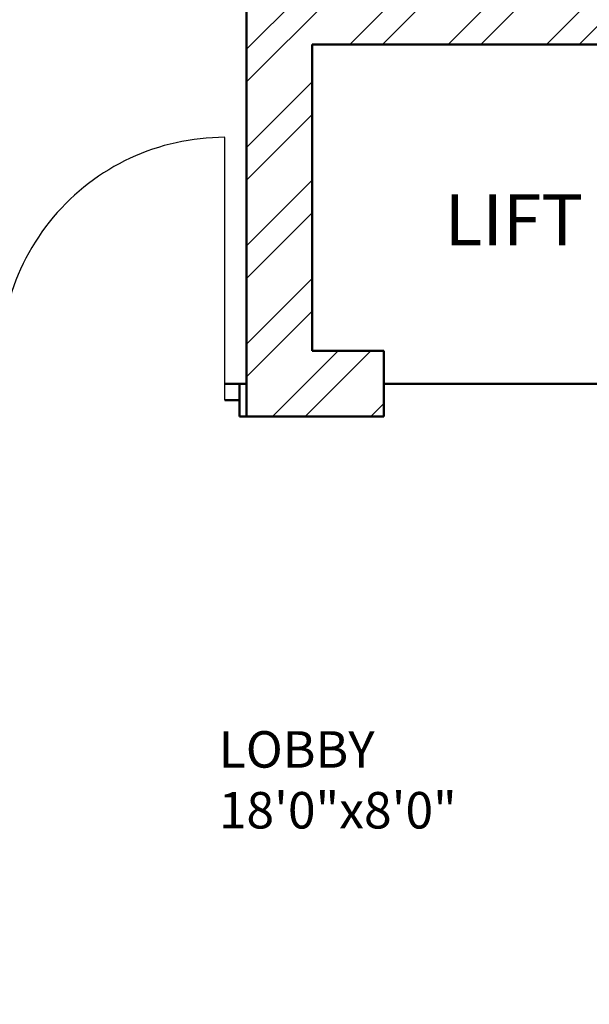
# Model space of a CAD drawing. Units: inches. Extents: x 1901 to 2863, y 888 to 2433.
# Tile 52 of 91: x 2303 to 2381, y 1732 to 1867. Entities that reach past the tile are written whole.
import ezdxf

# ---------------------------------------------------------------- set-up
doc = ezdxf.new("R2010")
doc.units = ezdxf.units.IN
for name, color, linetype, lineweight in [('A-AREA-IDEN', 7, 'Continuous', 18), ('A-DOOR', 4, 'Continuous', 25), ('A-WALL', 7, 'Continuous', 50), ('A-WALL-PATT', 8, 'Continuous', 13)]:
    doc.layers.add(name, color=color, linetype=linetype, lineweight=lineweight)
doc.styles.get("Standard").update_dxf_attribs({"font": 'arial.ttf'})

msp = doc.modelspace()

# ---------------------------------------------------------------- hatches: boundary and pattern name
at = {"layer": 'A-WALL-PATT'}
h = msp.add_hatch(dxfattribs=at)
h.set_pattern_fill('ANSI32', color=256)
h.paths.add_polyline_path([(2192.5, 2274.13), (2141.26, 2274.13), (2141.26, 2269.63), (2192.5, 2269.63)])
h.paths.add_polyline_path([(2259.93, 2274.13), (2216.5, 2274.13), (2216.5, 2269.63), (2255.43, 2269.63), (2255.43, 2214.63), (2250.81, 2214.63), (2250.81, 2210.13), (2259.93, 2210.13), (2259.93, 2215.13), (2271.76, 2215.13), (2271.76, 2217.38), (2271.76, 2219.63), (2259.93, 2219.63)])
h.paths.add_polyline_path([(2171.43, 2269.63), (2166.93, 2269.63), (2166.93, 2219.63), (2121.24, 2219.63), (2121.24, 2215.13), (2166.93, 2215.13), (2166.93, 2083.13), (2161.81, 2083.13), (2161.81, 2078.63), (2171.43, 2078.63), (2177, 2078.63), (2177, 2080.88), (2177, 2083.13), (2171.43, 2083.13), (2171.43, 2210.13), (2230.91, 2210.13), (2230.91, 2212.38), (2230.91, 2214.63), (2171.43, 2214.63)])
h.paths.add_polyline_path([(2117.26, 2274.13), (2089.43, 2274.13), (2089.43, 2219.63), (2081.14, 2219.63), (2081.14, 2215.13), (2089.43, 2215.13), (2098, 2215.13), (2098, 2217.38), (2098, 2219.63), (2093.93, 2219.63), (2093.93, 2269.63), (2117.26, 2269.63), (2117.26, 2271.88)])
h.paths.add_polyline_path([(2343.43, 2219.63), (2329.29, 2219.63), (2329.29, 2215.13), (2338.93, 2215.13), (2338.93, 2184.74), (2343.43, 2184.74)])
h.paths.add_polyline_path([(2338.93, 2083.13), (2329.29, 2083.13), (2208.97, 2083.13), (2208.97, 2078.63), (2338.93, 2078.63)])
h.paths.add_polyline_path([(2343.43, 2136.74), (2338.93, 2136.74), (2338.93, 1872.63), (2343.43, 1872.63)])
h.paths.add_polyline_path([(2343.43, 1863.63), (2397.68, 1863.63), (2397.68, 1821.63), (2384.14, 1821.63), (2384.14, 1812.63), (2418.33, 1812.63), (2418.33, 1817.13), (2418.33, 1821.63), (2406.68, 1821.63), (2406.68, 1863.63), (2459.5, 1863.63), (2459.5, 1821.63), (2447.14, 1821.63), (2447.14, 1812.63), (2459.5, 1812.63), (2468.5, 1812.63), (2468.5, 1872.63), (2394.43, 1872.63), (2334.43, 1872.63), (2334.43, 1812.63), (2343.43, 1812.63), (2353.25, 1812.63), (2353.25, 1821.63), (2343.43, 1821.63)])
h.paths.add_polyline_path([(2510.01, 1872.63), (2468.5, 1872.63), (2468.5, 1868.13), (2510.01, 1868.13)])
h.paths.add_polyline_path([(2514.01, 1817.13), (2468.5, 1817.13), (2468.5, 1812.63), (2482.11, 1812.63), (2482.11, 1800.61), (2486.61, 1800.61), (2486.61, 1812.63), (2514.01, 1812.63)])
h.paths.add_polyline_path([(2299.25, 1814.88), (2299.25, 1817.13), (2295.93, 1817.13), (2295.93, 1854.17), (2293.68, 1854.17), (2291.43, 1854.17), (2291.43, 1817.13), (2266.11, 1817.13), (2266.11, 1812.63), (2299.25, 1812.63)])
h.paths.add_polyline_path([(2218.11, 1817.13), (2206.46, 1817.13), (2171.43, 1817.13), (2171.43, 1949.13), (2190.1, 1949.13), (2190.1, 1953.63), (2163.47, 1953.63), (2163.47, 1949.13), (2166.93, 1949.13), (2166.93, 1817.13), (2114.3, 1817.13), (2114.3, 1812.63), (2218.11, 1812.63)])
h.paths.add_polyline_path([(2029.43, 1970.92), (2024.93, 1970.92), (2024.93, 1912.72), (2029.43, 1912.72)])
h.paths.add_polyline_path([(2132.3, 1953.63), (2113.93, 1953.63), (2113.93, 1975.89), (2111.68, 1975.89), (2109.43, 1975.89), (2109.43, 1953.63), (2029.43, 1953.63), (2029.43, 1949.13), (2132.3, 1949.13)])
h.paths.add_polyline_path([(2029.43, 1853.61), (2029.31, 1853.61), (2029.31, 1853.61), (2029.43, 1853.61), (2029.43, 1864.72), (2024.93, 1864.72), (2024.93, 1812.63), (2066.3, 1812.63), (2066.3, 1814.88), (2066.3, 1817.13), (2029.43, 1817.13)])
h.paths.add_polyline_path([(2122.93, 2010.09), (2120.68, 2010.09), (2118.43, 2010.09), (2118.43, 2006.13), (2029.43, 2006.13), (2029.43, 2001.63), (2109.43, 2001.63), (2109.43, 1998.04), (2113.93, 1998.04), (2113.93, 2001.63), (2122.93, 2001.63)])
h.paths.add_polyline_path([(2029.43, 2031.38), (2024.93, 2031.38), (2024.93, 1994.92), (2027.18, 1994.92), (2029.43, 1994.92)])
h.paths.add_polyline_path([(2029.43, 2136.74), (2024.93, 2136.74), (2024.93, 2067.38), (2027.18, 2067.38), (2029.43, 2067.38)])
h.paths.add_polyline_path([(2125.62, 2083.13), (2029.43, 2083.13), (2029.43, 2078.63), (2118.43, 2078.63), (2118.43, 2030.71), (2122.93, 2030.71), (2122.93, 2078.63), (2125.62, 2078.63)])
h.paths.add_polyline_path([(2029.43, 2215.13), (2040.47, 2215.13), (2040.47, 2217.38), (2040.47, 2219.63), (2024.93, 2219.63), (2024.93, 2184.74), (2029.43, 2184.74), (2029.43, 2187.78)])
h.paths.add_polyline_path([(2686.43, 2274.13), (2659.28, 2274.13), (2659.28, 2269.63), (2681.93, 2269.63), (2681.93, 2219.63), (2676.82, 2219.63), (2676.82, 2215.13), (2681.93, 2215.13), (2697.01, 2215.13), (2697.01, 2217.38), (2697.01, 2219.63), (2686.43, 2219.63)])
h.paths.add_polyline_path([(2609.93, 2269.63), (2635.28, 2269.63), (2635.28, 2274.13), (2571.43, 2274.13), (2571.43, 2269.63), (2605.43, 2269.63), (2605.43, 2214.63), (2549.1, 2214.63), (2549.1, 2210.13), (2605.43, 2210.13), (2605.43, 2083.13), (2601.01, 2083.13), (2601.01, 2080.88), (2601.01, 2078.63), (2609.93, 2078.63), (2616.16, 2078.63), (2616.16, 2080.88), (2616.16, 2083.13), (2609.93, 2083.13), (2609.93, 2215.13), (2651.46, 2215.13), (2651.46, 2217.38), (2651.46, 2219.63), (2609.93, 2219.63)])
h.paths.add_polyline_path([(2521.43, 2269.63), (2547.43, 2269.63), (2547.43, 2271.88), (2547.43, 2274.13), (2516.93, 2274.13), (2516.93, 2219.63), (2506.41, 2219.63), (2506.41, 2215.13), (2516.93, 2215.13), (2516.93, 2210.13), (2525.4, 2210.13), (2525.4, 2212.38), (2525.4, 2214.63), (2521.43, 2214.63)])
h.paths.add_polyline_path([(2456.01, 2219.63), (2439.43, 2219.63), (2439.43, 2187.89), (2443.93, 2187.89), (2443.93, 2215.13), (2456.01, 2215.13)])
h.paths.add_polyline_path([(2752.93, 2219.63), (2739.48, 2219.63), (2739.48, 2215.13), (2748.43, 2215.13), (2748.43, 2187.89), (2752.93, 2187.89)])
h.paths.add_polyline_path([(2752.93, 2139.89), (2748.43, 2139.89), (2748.43, 2083.13), (2648.42, 2083.13), (2648.42, 2078.63), (2654.93, 2078.63), (2654.93, 2039.44), (2659.43, 2039.44), (2659.43, 2078.63), (2748.43, 2078.63), (2748.43, 2063.43), (2752.93, 2063.43)])
h.paths.add_polyline_path([(2752.93, 2010.63), (2659.43, 2010.63), (2659.43, 2015.65), (2654.93, 2015.65), (2654.93, 2010.63), (2605.43, 2010.63), (2605.43, 1920.97), (2609.93, 1920.97), (2609.93, 2006.13), (2748.43, 2006.13), (2748.43, 1982.47), (2752.93, 1982.47)])
h.paths.add_polyline_path([(2752.93, 2027.43), (2748.43, 2027.43), (2748.43, 2010.63), (2752.93, 2010.63)])
h.paths.add_polyline_path([(2748.43, 1886.13), (2609.93, 1886.13), (2609.93, 1889.72), (2605.43, 1889.72), (2605.43, 1861.26), (2609.93, 1861.26), (2609.93, 1881.63), (2748.43, 1881.63)])
h.paths.add_polyline_path([(2456.86, 2228.83), (2498.4, 2228.83), (2498.4, 2247.49), (2456.86, 2247.49)], flags=9)
h.paths.add_polyline_path([(2038.6, 2237.42), (2080.17, 2237.42), (2080.17, 2256.08), (2038.6, 2256.08)], flags=9)
h.paths.add_polyline_path([(2292.01, 1062.39), (2539.93, 1062.39), (2539.93, 1099.49), (2292.01, 1099.49)], flags=9)
h.paths.add_polyline_path([(2424.91, 1832.25), (2448.51, 1832.25), (2448.51, 1846.68), (2424.91, 1846.68)], flags=25)
h.paths.add_polyline_path([(2359.08, 1832.25), (2382.68, 1832.25), (2382.68, 1846.68), (2359.08, 1846.68)], flags=25)
h.paths.add_polyline_path([(2352.9, 1684.8), (2367.54, 1684.8), (2367.54, 1697.17), (2352.9, 1697.17)], flags=9)
h.paths.add_polyline_path([(2079.29, 1755.83), (2169.02, 1755.83), (2169.02, 1774.37), (2079.29, 1774.37)], flags=9)
h.paths.add_polyline_path([(2404.09, 1373.86), (2404.09, 1463.59), (2385.54, 1463.59), (2385.54, 1373.86)], flags=9)
h.paths.add_polyline_path([(2268.09, 2236.37), (2309.64, 2236.37), (2309.64, 2255.03), (2268.09, 2255.03)], flags=9)
h.paths.add_polyline_path([(2575.96, 1700.95), (2665.7, 1700.95), (2665.7, 1719.5), (2575.96, 1719.5)], flags=9)
h.paths.add_polyline_path([(2302.96, 1878.47), (2329.52, 1878.47), (2329.52, 1888.78), (2302.96, 1888.78)], flags=9)
h.paths.add_polyline_path([(2097.42, 2240.58), (2126.57, 2240.58), (2126.57, 2259.23), (2097.42, 2259.23)], flags=9)
h.paths.add_polyline_path([(2208.72, 2246.12), (2237.88, 2246.12), (2237.88, 2264.78), (2208.72, 2264.78)], flags=9)
h.paths.add_polyline_path([(2038.15, 1925.96), (2076.99, 1925.96), (2076.99, 1944.62), (2038.15, 1944.62)], flags=9)
h.paths.add_polyline_path([(2239.14, 1926.67), (2288.46, 1926.67), (2288.46, 1945.33), (2239.14, 1945.33)], flags=9)
h.paths.add_polyline_path([(2175.43, 2007.33), (2212.36, 2007.33), (2212.36, 2025.99), (2175.43, 2025.99)], flags=9)
h.paths.add_polyline_path([(2225.03, 2091.79), (2263.87, 2091.79), (2263.87, 2110.45), (2225.03, 2110.45)], flags=9)
h.paths.add_polyline_path([(2035.4, 2098.48), (2074.24, 2098.48), (2074.24, 2117.14), (2035.4, 2117.14)], flags=9)
h.paths.add_polyline_path([(2050.1, 2029.21), (2083.26, 2029.21), (2083.26, 2047.87), (2050.1, 2047.87)], flags=9)
h.paths.add_polyline_path([(2069.68, 1956.72), (2098.83, 1956.72), (2098.83, 1975.38), (2069.68, 1975.38)], flags=25)
h.paths.add_polyline_path([(2328.62, 1753.34), (2361.66, 1753.34), (2361.66, 1771.99), (2328.62, 1771.99)], flags=9)
h.paths.add_polyline_path([(2395.16, 2060.89), (2395.16, 2140.65), (2378.68, 2140.65), (2378.68, 2060.89)], flags=9)
h.paths.add_polyline_path([(2463.73, 2059.02), (2492.89, 2059.02), (2492.89, 2077.68), (2463.73, 2077.68)], flags=9)
h.paths.add_polyline_path([(2458.03, 2181.54), (2496.87, 2181.54), (2496.87, 2200.19), (2458.03, 2200.19)], flags=9)
h.paths.add_polyline_path([(2527.58, 2243.07), (2556.73, 2243.07), (2556.73, 2261.73), (2527.58, 2261.73)], flags=9)
h.paths.add_polyline_path([(2694.46, 2232.77), (2736.03, 2232.77), (2736.03, 2251.42), (2694.46, 2251.42)], flags=9)
h.paths.add_polyline_path([(2637.82, 2249.22), (2666.98, 2249.22), (2666.98, 2267.88), (2637.82, 2267.88)], flags=9)
h.paths.add_polyline_path([(2623.69, 2183.54), (2662.53, 2183.54), (2662.53, 2202.2), (2623.69, 2202.2)], flags=9)
h.paths.add_polyline_path([(2691.97, 2021.5), (2725.12, 2021.5), (2725.12, 2040.16), (2691.97, 2040.16)], flags=9)
h.paths.add_polyline_path([(2621.04, 1975.91), (2662.34, 1975.91), (2662.34, 1994.57), (2621.04, 1994.57)], flags=25)
h.paths.add_polyline_path([(2479.03, 1927.62), (2519.84, 1927.62), (2519.84, 1946.28), (2479.03, 1946.28)], flags=9)
h.paths.add_polyline_path([(2670.94, 1849.08), (2716.01, 1849.08), (2716.01, 1867.73), (2670.94, 1867.73)], flags=9)
h.paths.add_polyline_path([(2523.61, 1782.96), (2550.17, 1782.96), (2550.17, 1793.26), (2523.61, 1793.26)], flags=9)
h.paths.add_polyline_path([(2450.84, 1207.33), (2492.39, 1207.33), (2492.39, 1225.99), (2450.84, 1225.99)], flags=9)
h.paths.add_polyline_path([(2527.75, 1203.84), (2556.91, 1203.84), (2556.91, 1222.5), (2527.75, 1222.5)], flags=9)
h.paths.add_polyline_path([(2639.11, 1207.2), (2668.27, 1207.2), (2668.27, 1225.86), (2639.11, 1225.86)], flags=9)
h.paths.add_polyline_path([(2692.59, 1218.97), (2734.17, 1218.97), (2734.17, 1237.62), (2692.59, 1237.62)], flags=9)
h.paths.add_polyline_path([(2669.27, 1366.33), (2708.11, 1366.33), (2708.11, 1384.99), (2669.27, 1384.99)], flags=9)
h.paths.add_polyline_path([(2463.31, 1358.03), (2502.15, 1358.03), (2502.15, 1376.69), (2463.31, 1376.69)], flags=9)
h.paths.add_polyline_path([(2494.72, 1449.96), (2531.65, 1449.96), (2531.65, 1468.62), (2494.72, 1468.62)], flags=9)
h.paths.add_polyline_path([(2675.57, 1422.16), (2708.72, 1422.16), (2708.72, 1440.81), (2675.57, 1440.81)], flags=9)
h.paths.add_polyline_path([(2685.63, 1493.89), (2714.79, 1493.89), (2714.79, 1512.55), (2685.63, 1512.55)], flags=9)
h.paths.add_polyline_path([(2686.8, 1529.91), (2725.65, 1529.91), (2725.65, 1548.57), (2686.8, 1548.57)], flags=9)
h.paths.add_polyline_path([(2503.65, 1537.99), (2552.97, 1537.99), (2552.97, 1556.65), (2503.65, 1556.65)], flags=9)
h.paths.add_polyline_path([(2291.71, 1643.5), (2318.28, 1643.5), (2318.28, 1653.81), (2291.71, 1653.81)], flags=9)
h.paths.add_polyline_path([(2450.63, 1610.52), (2477.19, 1610.52), (2477.19, 1620.82), (2450.63, 1620.82)], flags=9)
h.paths.add_polyline_path([(2359.99, 1551.81), (2422.25, 1551.81), (2422.25, 1562.12), (2359.99, 1562.12)], flags=9)
h.paths.add_polyline_path([(2280.11, 1249.01), (2321.65, 1249.01), (2321.65, 1267.66), (2280.11, 1267.66)], flags=9)
h.paths.add_polyline_path([(2164.06, 1274.23), (2193.22, 1274.23), (2193.22, 1292.89), (2164.06, 1292.89)], flags=9)
h.paths.add_polyline_path([(2118.21, 1277.69), (2151.25, 1277.69), (2151.25, 1296.35), (2118.21, 1296.35)], flags=9)
h.paths.add_polyline_path([(2031.95, 1268.53), (2073.52, 1268.53), (2073.52, 1287.19), (2031.95, 1287.19)], flags=9)
h.paths.add_polyline_path([(2050.2, 1409.08), (2089.04, 1409.08), (2089.04, 1427.74), (2050.2, 1427.74)], flags=9)
h.paths.add_polyline_path([(2243.74, 1421.03), (2282.58, 1421.03), (2282.58, 1439.69), (2243.74, 1439.69)], flags=9)
h.paths.add_polyline_path([(2190.75, 1509.77), (2231.56, 1509.77), (2231.56, 1528.43), (2190.75, 1528.43)], flags=9)
h.paths.add_polyline_path([(2058.39, 1475.42), (2091.55, 1475.42), (2091.55, 1494.07), (2058.39, 1494.07)], flags=9)
h.paths.add_polyline_path([(2062.45, 1553.09), (2091.6, 1553.09), (2091.6, 1571.75), (2062.45, 1571.75)], flags=9)
h.paths.add_polyline_path([(2219.52, 1590.37), (2266.15, 1590.37), (2266.15, 1609.02), (2219.52, 1609.02)], flags=9)
h.paths.add_polyline_path([(2041.07, 1584.19), (2079.91, 1584.19), (2079.91, 1602.85), (2041.07, 1602.85)], flags=9)
h = msp.add_hatch(dxfattribs=at)
h.set_pattern_fill('ANSI32', color=256)
h.paths.add_polyline_path([(2443.93, 2139.89), (2439.43, 2139.89), (2439.43, 2069.35), (2441.68, 2069.35), (2443.93, 2069.35), (2443.93, 2078.63), (2521.93, 2078.63), (2521.93, 2075.07), (2524.18, 2075.07), (2526.43, 2075.07), (2526.43, 2078.63), (2571.75, 2078.63), (2571.75, 2080.88), (2571.75, 2083.13), (2443.93, 2083.13)])
h.paths.add_polyline_path([(2526.43, 2054.63), (2524.18, 2054.63), (2521.93, 2054.63), (2521.93, 2030.63), (2443.93, 2030.63), (2443.93, 2045.35), (2439.43, 2045.35), (2439.43, 1983.87), (2443.93, 1983.87), (2443.93, 2026.13), (2521.93, 2026.13), (2526.43, 2026.13)])
h.paths.add_polyline_path([(2443.93, 1923.87), (2439.43, 1923.87), (2439.43, 1872.63), (2443.93, 1872.63)])
h.paths.add_polyline_path([(2636.23, 1766.13), (2609.93, 1766.13), (2609.93, 1779.79), (2605.43, 1779.79), (2605.43, 1766.13), (2486.61, 1766.13), (2486.61, 1770.67), (2482.11, 1770.67), (2482.11, 1766.13), (2482.11, 1761.63), (2636.23, 1761.63), (2636.23, 1763.88)])
h.paths.add_polyline_path([(2519.54, 1663.38), (2519.54, 1665.63), (2494.93, 1665.63), (2481.83, 1665.63), (2481.83, 1663.38), (2481.83, 1661.13), (2490.43, 1661.13), (2490.43, 1640.16), (2494.93, 1640.16), (2494.93, 1661.13), (2519.54, 1661.13)])
h.paths.add_polyline_path([(2443.93, 1712.13), (2443.93, 1716.63), (2414.46, 1716.63), (2414.46, 1712.13), (2439.43, 1712.13), (2439.43, 1545.51), (2443.93, 1545.51), (2443.93, 1661.13), (2448.47, 1661.13), (2448.47, 1665.63), (2443.93, 1665.63)])
h.paths.add_polyline_path([(2343.43, 1712.13), (2365.52, 1712.13), (2365.52, 1714.38), (2365.52, 1716.63), (2333.87, 1716.63), (2333.87, 1714.38), (2333.87, 1712.13), (2338.93, 1712.13), (2338.93, 1575.63), (2338.93, 1545.51), (2343.43, 1545.51), (2343.43, 1547.51), (2343.43, 1580.13)])
h.paths.add_polyline_path([(2752.93, 1665.63), (2579.54, 1665.63), (2579.54, 1661.13), (2615.93, 1661.13), (2615.93, 1529.13), (2598.93, 1529.13), (2598.93, 1524.63), (2623.13, 1524.63), (2623.13, 1526.88), (2623.13, 1529.13), (2620.43, 1529.13), (2620.43, 1661.13), (2748.43, 1661.13), (2748.43, 1633.5), (2752.93, 1633.5)])
h.paths.add_polyline_path([(2752.93, 1419.93), (2748.43, 1419.93), (2748.43, 1400.13), (2659.43, 1400.13), (2659.43, 1444.33), (2657.18, 1444.33), (2654.93, 1444.33), (2654.93, 1400.13), (2643.65, 1400.13), (2643.65, 1395.63), (2748.43, 1395.63), (2748.43, 1364.04), (2752.93, 1364.04)])
h.paths.add_polyline_path([(2752.93, 1492.88), (2748.43, 1492.88), (2748.43, 1476.63), (2667.43, 1476.63), (2667.43, 1479.71), (2665.18, 1479.71), (2662.93, 1479.71), (2662.93, 1476.63), (2654.93, 1476.63), (2654.93, 1469.54), (2659.43, 1469.54), (2659.43, 1472.13), (2748.43, 1472.13), (2748.43, 1455.93), (2752.93, 1455.93)])
h.paths.add_polyline_path([(2752.93, 1304.04), (2748.43, 1304.04), (2748.43, 1263.63), (2738.66, 1263.63), (2738.66, 1259.13), (2752.93, 1259.13)])
h.paths.add_polyline_path([(2685.93, 1259.13), (2695.49, 1259.13), (2695.49, 1261.38), (2695.49, 1263.63), (2677.84, 1263.63), (2677.84, 1261.38), (2677.84, 1259.13), (2681.43, 1259.13), (2681.43, 1203.63), (2653.28, 1203.63), (2653.28, 1199.13), (2685.93, 1199.13), (2685.93, 1203.63)])
h.paths.add_polyline_path([(2609.43, 1395.63), (2611.85, 1395.63), (2611.85, 1400.13), (2598.89, 1400.13), (2598.89, 1397.88), (2598.89, 1395.63), (2604.93, 1395.63), (2604.93, 1268.13), (2554.73, 1268.13), (2554.73, 1265.88), (2554.73, 1263.63), (2604.93, 1263.63), (2604.93, 1203.63), (2571.31, 1203.63), (2571.31, 1199.13), (2604.93, 1199.13), (2629.28, 1199.13), (2629.28, 1201.38), (2629.28, 1203.63), (2609.43, 1203.63), (2609.43, 1258.63), (2609.43, 1259.13), (2654.8, 1259.13), (2654.8, 1263.63), (2609.43, 1263.63)])
h.paths.add_polyline_path([(2443.93, 1304.04), (2439.43, 1304.04), (2439.43, 1259.13), (2443.93, 1259.13), (2456.16, 1259.13), (2456.16, 1261.38), (2456.16, 1263.63), (2443.93, 1263.63)])
h.paths.add_polyline_path([(2525.43, 1263.63), (2531.78, 1263.63), (2531.78, 1268.13), (2520.93, 1268.13), (2520.93, 1263.63), (2511.41, 1263.63), (2511.41, 1259.13), (2520.93, 1259.13), (2520.93, 1199.13), (2547.31, 1199.13), (2547.31, 1201.38), (2547.31, 1203.63), (2525.43, 1203.63)])
h.paths.add_polyline_path([(2443.93, 1434.84), (2439.43, 1434.84), (2439.43, 1364.04), (2441.68, 1364.04), (2443.93, 1364.04)])
h.paths.add_polyline_path([(2567.13, 1400.13), (2443.93, 1400.13), (2443.93, 1395.63), (2567.13, 1395.63)])
h.paths.add_polyline_path([(2443.93, 1545.51), (2439.43, 1545.51), (2439.43, 1494.84), (2443.93, 1494.84)])
h.paths.add_polyline_path([(2494.93, 1553.35), (2492.68, 1553.35), (2490.43, 1553.35), (2490.43, 1524.63), (2494.93, 1524.63), (2525.94, 1524.63), (2525.94, 1526.88), (2525.94, 1529.13), (2494.93, 1529.13)])
h.paths.add_polyline_path([(2752.93, 1573.5), (2748.43, 1573.5), (2748.43, 1529.13), (2657.76, 1529.13), (2657.76, 1524.63), (2662.93, 1524.63), (2662.93, 1498.63), (2667.43, 1498.63), (2667.43, 1524.63), (2748.43, 1524.63), (2748.43, 1516.88), (2752.93, 1516.88)])
h.paths.add_polyline_path([(2038.6, 2237.42), (2080.17, 2237.42), (2080.17, 2256.08), (2038.6, 2256.08)], flags=9)
h.paths.add_polyline_path([(2292.01, 1062.39), (2539.93, 1062.39), (2539.93, 1099.49), (2292.01, 1099.49)], flags=9)
h.paths.add_polyline_path([(2424.91, 1832.25), (2448.51, 1832.25), (2448.51, 1846.68), (2424.91, 1846.68)], flags=9)
h.paths.add_polyline_path([(2359.08, 1832.25), (2382.68, 1832.25), (2382.68, 1846.68), (2359.08, 1846.68)], flags=9)
h.paths.add_polyline_path([(2352.9, 1684.8), (2367.54, 1684.8), (2367.54, 1697.17), (2352.9, 1697.17)], flags=9)
h.paths.add_polyline_path([(2079.29, 1755.83), (2169.02, 1755.83), (2169.02, 1774.37), (2079.29, 1774.37)], flags=9)
h.paths.add_polyline_path([(2404.09, 1373.86), (2404.09, 1463.59), (2385.54, 1463.59), (2385.54, 1373.86)], flags=9)
h.paths.add_polyline_path([(2268.09, 2236.37), (2309.64, 2236.37), (2309.64, 2255.03), (2268.09, 2255.03)], flags=9)
h.paths.add_polyline_path([(2575.96, 1700.95), (2665.7, 1700.95), (2665.7, 1719.5), (2575.96, 1719.5)], flags=9)
h.paths.add_polyline_path([(2302.96, 1878.47), (2329.52, 1878.47), (2329.52, 1888.78), (2302.96, 1888.78)], flags=9)
h.paths.add_polyline_path([(2097.42, 2240.58), (2126.57, 2240.58), (2126.57, 2259.23), (2097.42, 2259.23)], flags=9)
h.paths.add_polyline_path([(2208.72, 2246.12), (2237.88, 2246.12), (2237.88, 2264.78), (2208.72, 2264.78)], flags=9)
h.paths.add_polyline_path([(2038.15, 1925.96), (2076.99, 1925.96), (2076.99, 1944.62), (2038.15, 1944.62)], flags=9)
h.paths.add_polyline_path([(2239.14, 1926.67), (2288.46, 1926.67), (2288.46, 1945.33), (2239.14, 1945.33)], flags=9)
h.paths.add_polyline_path([(2175.43, 2007.33), (2212.36, 2007.33), (2212.36, 2025.99), (2175.43, 2025.99)], flags=9)
h.paths.add_polyline_path([(2225.03, 2091.79), (2263.87, 2091.79), (2263.87, 2110.45), (2225.03, 2110.45)], flags=9)
h.paths.add_polyline_path([(2035.4, 2098.48), (2074.24, 2098.48), (2074.24, 2117.14), (2035.4, 2117.14)], flags=9)
h.paths.add_polyline_path([(2050.1, 2029.21), (2083.26, 2029.21), (2083.26, 2047.87), (2050.1, 2047.87)], flags=9)
h.paths.add_polyline_path([(2069.68, 1956.72), (2098.83, 1956.72), (2098.83, 1975.38), (2069.68, 1975.38)], flags=9)
h.paths.add_polyline_path([(2328.62, 1753.34), (2361.66, 1753.34), (2361.66, 1771.99), (2328.62, 1771.99)], flags=9)
h.paths.add_polyline_path([(2395.16, 2060.89), (2395.16, 2140.65), (2378.68, 2140.65), (2378.68, 2060.89)], flags=9)
h.paths.add_polyline_path([(2463.73, 2059.02), (2492.89, 2059.02), (2492.89, 2077.68), (2463.73, 2077.68)], flags=9)
h.paths.add_polyline_path([(2458.03, 2181.54), (2496.87, 2181.54), (2496.87, 2200.19), (2458.03, 2200.19)], flags=9)
h.paths.add_polyline_path([(2456.86, 2228.83), (2498.4, 2228.83), (2498.4, 2247.49), (2456.86, 2247.49)], flags=9)
h.paths.add_polyline_path([(2527.58, 2243.07), (2556.73, 2243.07), (2556.73, 2261.73), (2527.58, 2261.73)], flags=9)
h.paths.add_polyline_path([(2694.46, 2232.77), (2736.03, 2232.77), (2736.03, 2251.42), (2694.46, 2251.42)], flags=9)
h.paths.add_polyline_path([(2637.82, 2249.22), (2666.98, 2249.22), (2666.98, 2267.88), (2637.82, 2267.88)], flags=9)
h.paths.add_polyline_path([(2623.69, 2183.54), (2662.53, 2183.54), (2662.53, 2202.2), (2623.69, 2202.2)], flags=9)
h.paths.add_polyline_path([(2691.97, 2021.5), (2725.12, 2021.5), (2725.12, 2040.16), (2691.97, 2040.16)], flags=9)
h.paths.add_polyline_path([(2621.04, 1975.91), (2662.34, 1975.91), (2662.34, 1994.57), (2621.04, 1994.57)], flags=9)
h.paths.add_polyline_path([(2479.03, 1927.62), (2519.84, 1927.62), (2519.84, 1946.28), (2479.03, 1946.28)], flags=9)
h.paths.add_polyline_path([(2670.94, 1849.08), (2716.01, 1849.08), (2716.01, 1867.73), (2670.94, 1867.73)], flags=9)
h.paths.add_polyline_path([(2523.61, 1782.96), (2550.17, 1782.96), (2550.17, 1793.26), (2523.61, 1793.26)], flags=9)
h.paths.add_polyline_path([(2450.84, 1207.33), (2492.39, 1207.33), (2492.39, 1225.99), (2450.84, 1225.99)], flags=9)
h.paths.add_polyline_path([(2527.75, 1203.84), (2556.91, 1203.84), (2556.91, 1222.5), (2527.75, 1222.5)], flags=9)
h.paths.add_polyline_path([(2639.11, 1207.2), (2668.27, 1207.2), (2668.27, 1225.86), (2639.11, 1225.86)], flags=9)
h.paths.add_polyline_path([(2692.59, 1218.97), (2734.17, 1218.97), (2734.17, 1237.62), (2692.59, 1237.62)], flags=9)
h.paths.add_polyline_path([(2669.27, 1366.33), (2708.11, 1366.33), (2708.11, 1384.99), (2669.27, 1384.99)], flags=25)
h.paths.add_polyline_path([(2463.31, 1358.03), (2502.15, 1358.03), (2502.15, 1376.69), (2463.31, 1376.69)], flags=9)
h.paths.add_polyline_path([(2494.72, 1449.96), (2531.65, 1449.96), (2531.65, 1468.62), (2494.72, 1468.62)], flags=9)
h.paths.add_polyline_path([(2675.57, 1422.16), (2708.72, 1422.16), (2708.72, 1440.81), (2675.57, 1440.81)], flags=25)
h.paths.add_polyline_path([(2685.63, 1493.89), (2714.79, 1493.89), (2714.79, 1512.55), (2685.63, 1512.55)], flags=9)
h.paths.add_polyline_path([(2686.8, 1529.91), (2725.65, 1529.91), (2725.65, 1548.57), (2686.8, 1548.57)], flags=25)
h.paths.add_polyline_path([(2503.65, 1537.99), (2552.97, 1537.99), (2552.97, 1556.65), (2503.65, 1556.65)], flags=9)
h.paths.add_polyline_path([(2291.71, 1643.5), (2318.28, 1643.5), (2318.28, 1653.81), (2291.71, 1653.81)], flags=9)
h.paths.add_polyline_path([(2450.63, 1610.52), (2477.19, 1610.52), (2477.19, 1620.82), (2450.63, 1620.82)], flags=9)
h.paths.add_polyline_path([(2359.99, 1551.81), (2422.25, 1551.81), (2422.25, 1562.12), (2359.99, 1562.12)], flags=9)
h.paths.add_polyline_path([(2280.11, 1249.01), (2321.65, 1249.01), (2321.65, 1267.66), (2280.11, 1267.66)], flags=9)
h.paths.add_polyline_path([(2164.06, 1274.23), (2193.22, 1274.23), (2193.22, 1292.89), (2164.06, 1292.89)], flags=9)
h.paths.add_polyline_path([(2118.21, 1277.69), (2151.25, 1277.69), (2151.25, 1296.35), (2118.21, 1296.35)], flags=9)
h.paths.add_polyline_path([(2031.95, 1268.53), (2073.52, 1268.53), (2073.52, 1287.19), (2031.95, 1287.19)], flags=9)
h.paths.add_polyline_path([(2050.2, 1409.08), (2089.04, 1409.08), (2089.04, 1427.74), (2050.2, 1427.74)], flags=9)
h.paths.add_polyline_path([(2243.74, 1421.03), (2282.58, 1421.03), (2282.58, 1439.69), (2243.74, 1439.69)], flags=9)
h.paths.add_polyline_path([(2190.75, 1509.77), (2231.56, 1509.77), (2231.56, 1528.43), (2190.75, 1528.43)], flags=9)
h.paths.add_polyline_path([(2058.39, 1475.42), (2091.55, 1475.42), (2091.55, 1494.07), (2058.39, 1494.07)], flags=9)
h.paths.add_polyline_path([(2062.45, 1553.09), (2091.6, 1553.09), (2091.6, 1571.75), (2062.45, 1571.75)], flags=9)
h.paths.add_polyline_path([(2219.52, 1590.37), (2266.15, 1590.37), (2266.15, 1609.02), (2219.52, 1609.02)], flags=9)
h.paths.add_polyline_path([(2041.07, 1584.19), (2079.91, 1584.19), (2079.91, 1602.85), (2041.07, 1602.85)], flags=9)

# ---------------------------------------------------------------- linework, layer by layer
at = {"layer": 'A-DOOR'}
msp.add_line((2331.45, 1814.88), (2331.45, 1850.88), dxfattribs=at)
msp.add_arc((2331.45, 1820.22), 30.67, 90, 190.0141, dxfattribs=at)
at = {"layer": 'A-WALL'}
for p, q in [((2334.43, 1812.63), (2334.43, 1872.63)), ((2343.43, 1863.63), (2343.43, 1821.63)), ((2397.68, 1863.63), (2343.43, 1863.63)), ((2343.43, 1821.63), (2343.43, 1821.63)), ((2353.25, 1821.63), (2343.43, 1821.63)), ((2353.25, 1821.63), (2353.25, 1812.63)), ((2331.45, 1817.13), (2334.43, 1817.13)), ((2333.45, 1817.13), (2333.45, 1812.63)), ((2384.14, 1817.13), (2353.25, 1817.13)), ((2333.45, 1814.88), (2331.45, 1814.88)), ((2333.45, 1812.63), (2333.45, 1814.88)), ((2333.45, 1812.63), (2343.43, 1812.63)), ((2343.43, 1812.63), (2334.43, 1812.63)), ((2343.43, 1812.63), (2353.25, 1812.63))]:
    msp.add_line(p, q, dxfattribs=at)

# ---------------------------------------------------------------- texts
at = {"layer": 'A-AREA-IDEN', "attachment_point": 1}
for s, width, insert, char_height in [('LIFT', 68.4851, (2361.54, 1843.08), 7), ('LOBBY\\P18\'0"x8\'0"', 155.9829, (2330.63, 1769.51), 5)]:
    msp.add_mtext_dynamic_manual_height_columns(s, width=width, gutter_width=12.5, heights=[0], dxfattribs=dict(at, insert=insert, char_height=char_height))

doc.saveas('drawing.dxf')
